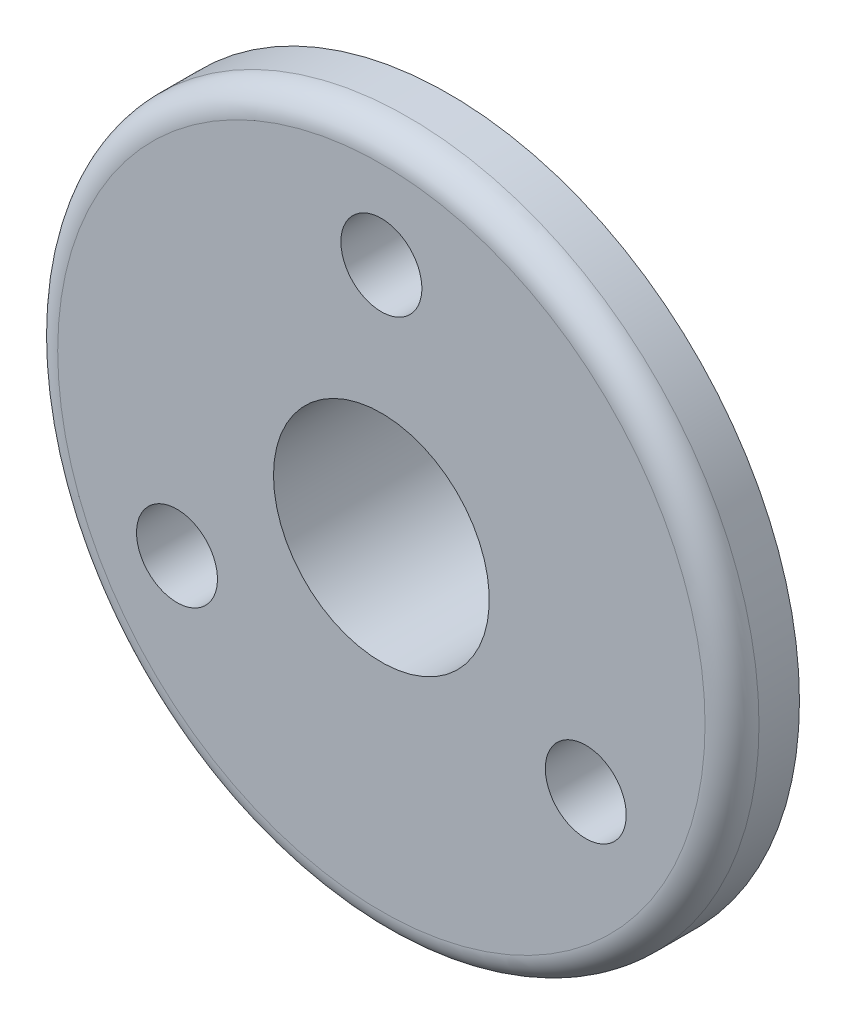
from build123d import *

# Parameters (mm, degrees)
FLANGE_PROFILE_R                 = 26
FLANGE_52_DEPTH                  = 5
HUB_PROFILE_R                    = 12.5
HUB_25_DEPTH                     = 7
BORE_16_DEPTH                    = 39.678159212
BORE_16_DEPTH_BACK               = 39.678159212
BORE_PROFILE_R                   = 8
BOLT_HOLES_3X_6_PCD35_DEPTH      = 38.429934544
BOLT_HOLES_3X_6_PCD35_DEPTH_BACK = 38.429934544
BOLT_HOLE_PROFILE_R              = 3
FLANGE_EDGE_FILLET_R2_R          = 2


with BuildPart() as part:
    # Flange Profile → Flange Ø52 (new body)
    with BuildSketch(Plane.XY):
        Circle(FLANGE_PROFILE_R)
    extrude(amount=-FLANGE_52_DEPTH)

    # Hub Profile → Hub Ø25 (add)
    with BuildSketch(Plane(origin=(0, 0, -5), x_dir=(-1, 0, 0), z_dir=(0, 0, -1))):
        Circle(HUB_PROFILE_R)
    extrude(amount=HUB_25_DEPTH)

    # Bore Profile → Bore Ø16 (cut, two sides: drawn at the far end of the back side and taken through both)
    with BuildSketch(Plane(origin=(0, 0, -12), x_dir=(-1, 0, 0), z_dir=(0, 0, -1)).offset(-BORE_16_DEPTH_BACK)):
        Circle(BORE_PROFILE_R)
    extrude(amount=BORE_16_DEPTH + BORE_16_DEPTH_BACK, mode=Mode.SUBTRACT)

    # Bolt Hole Profile → Bolt Holes 3xØ6 PCD35 (cut, two sides: drawn at the far end of the back side and taken through both)
    with BuildSketch(Plane(origin=(0, 0, -5), x_dir=(-1, 0, 0), z_dir=(0, 0, -1)).offset(-BOLT_HOLES_3X_6_PCD35_DEPTH_BACK)):
        with Locations((0, 17.5)):
            Circle(BOLT_HOLE_PROFILE_R)
        with Locations((15.155444566, -8.75)):
            Circle(BOLT_HOLE_PROFILE_R)
        with Locations((-15.155444566, -8.75)):
            Circle(BOLT_HOLE_PROFILE_R)
    extrude(amount=BOLT_HOLES_3X_6_PCD35_DEPTH + BOLT_HOLES_3X_6_PCD35_DEPTH_BACK, mode=Mode.SUBTRACT)

    # Flange Edge Fillet R2
    flange_edge_fillet_r2_edges = [part.edges().sort_by_distance(p)[0] for p in [
        (-26, 0, 0),
    ]]
    fillet(flange_edge_fillet_r2_edges, radius=FLANGE_EDGE_FILLET_R2_R)


solid = part.part
